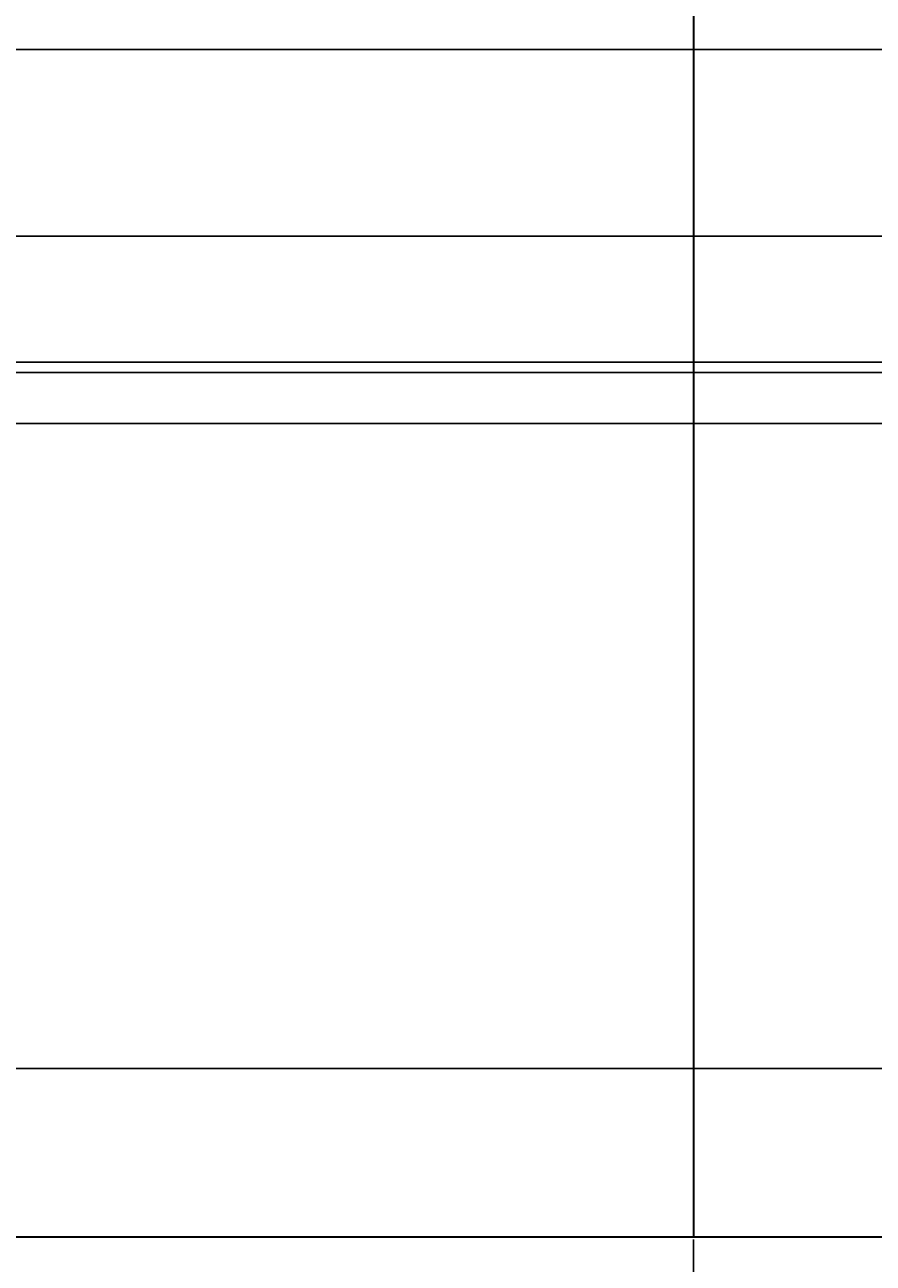
# Model space of a CAD drawing. Units: inches. Extents: x 27 to 200, y -50 to 102.
# Tile 4 of 26: x 67 to 89, y -17 to 15. Entities that reach past the tile are written whole.
import ezdxf

# ---------------------------------------------------------------- set-up
doc = ezdxf.new("R2010")
doc.units = ezdxf.units.IN
doc.header["$MEASUREMENT"] = 0
doc.layers.add('A-ANNO-DIMS', color=2, linetype='Continuous', lineweight=18)
doc.layers.add('A-ELEV', color=7, linetype='Continuous', lineweight=35)
doc.styles.get("Standard").update_dxf_attribs({"font": 'arial.ttf'})
doc.dimstyles.get("Standard").update_dxf_attribs({"dimtxt": 0.18, "dimasz": 0.18, "dimexe": 0.18, "dimexo": 0.0625, "dimgap": 0.09, "dimtad": 0, "dimtih": 1, "dimtoh": 1, "dimdec": 4, "dimzin": 0, "dimdsep": 46, "dimtxsty": 'Standard', "dimcen": 0.09, "dimadec": 0, "dimazin": 0, "dimtfac": 1, "dimtdec": 4, "dimtofl": 0, "dimtmove": 0, "dimatfit": 3, "dimfxl": 1, "dimtolj": 1, "dimtzin": 0, "dimarcsym": 0})

# ---------------------------------------------------------------- blocks, each defined once
blk = doc.blocks.new('*D23')
at = {"layer": 'A-ANNO-DIMS', "color": 0, "lineweight": -2, "transparency": 16777216}
for p, q in [((35.417, -16.832), (35.417, -25.149)), ((191.417, -16.832), (191.417, -25.149)), ((35.597, -24.969), (113.137, -24.969)), ((191.237, -24.969), (113.697, -24.969))]:
    blk.add_line(p, q, dxfattribs=at)
at = {"layer": 'A-ANNO-DIMS', "color": 0, "transparency": 16777216}
for points in [[(35.597, -24.939), (35.597, -24.999), (35.417, -24.969)], [(191.237, -24.939), (191.237, -24.999), (191.417, -24.969)]]:
    blk.add_solid(points, dxfattribs=at)
at = {"layer": 'Defpoints', "color": 0, "transparency": 16777216}
for p in [(35.417, -16.769), (191.417, -16.769), (191.417, -24.969)]:
    blk.add_point(p, dxfattribs=at)
at = {"layer": 'A-ANNO-DIMS', "color": 0, "transparency": 16777216, "insert": (113.417, -24.969), "char_height": 0.18, "attachment_point": 5}
blk.add_mtext('\\A1;156', dxfattribs=at)
blk = doc.blocks.new('*D33')
at = {"layer": 'A-ANNO-DIMS', "color": 0, "lineweight": -2, "transparency": 16777216}
for p, q in [((84.417, -16.832), (84.417, -25.149)), ((89.312, -16.832), (89.312, -25.149)), ((84.597, -24.969), (86.466, -24.969)), ((89.132, -24.969), (87.262, -24.969))]:
    blk.add_line(p, q, dxfattribs=at)
at = {"layer": 'A-ANNO-DIMS', "color": 0, "transparency": 16777216}
for points in [[(84.597, -24.939), (84.597, -24.999), (84.417, -24.969)], [(89.132, -24.939), (89.132, -24.999), (89.312, -24.969)]]:
    blk.add_solid(points, dxfattribs=at)
at = {"layer": 'Defpoints', "color": 0, "transparency": 16777216}
for p in [(84.417, -16.769), (89.312, -16.769), (89.312, -24.969)]:
    blk.add_point(p, dxfattribs=at)
at = {"layer": 'A-ANNO-DIMS', "color": 0, "transparency": 16777216, "insert": (86.864, -24.969), "char_height": 0.18, "attachment_point": 5}
blk.add_mtext('\\A1;4.895', dxfattribs=at)
blk = doc.blocks.new('*D43')
at = {"layer": 'A-ANNO-DIMS', "color": 0, "lineweight": -2, "transparency": 16777216}
for p, q in [((66.479, -3.679), (66.479, -25.149)), ((84.417, -16.832), (84.417, -25.149)), ((66.659, -24.969), (75.063, -24.969)), ((84.237, -24.969), (75.833, -24.969))]:
    blk.add_line(p, q, dxfattribs=at)
at = {"layer": 'A-ANNO-DIMS', "color": 0, "transparency": 16777216}
for points in [[(66.659, -24.939), (66.659, -24.999), (66.479, -24.969)], [(84.237, -24.939), (84.237, -24.999), (84.417, -24.969)]]:
    blk.add_solid(points, dxfattribs=at)
at = {"layer": 'Defpoints', "color": 0, "transparency": 16777216}
for p in [(66.479, -3.617), (84.417, -16.769), (84.417, -24.969)]:
    blk.add_point(p, dxfattribs=at)
at = {"layer": 'A-ANNO-DIMS', "color": 0, "transparency": 16777216, "insert": (75.448, -24.969), "char_height": 0.18, "attachment_point": 5}
blk.add_mtext('\\A1;17.94', dxfattribs=at)
blk = doc.blocks.new('*D48')
at = {"layer": 'A-ANNO-DIMS', "color": 0, "lineweight": -2, "transparency": 16777216}
for p, q in [((84.479, 44.926), (199.797, 44.926)), ((199.617, 44.746), (199.617, 14.26)), ((199.617, -16.589), (199.617, 13.897)), ((84.479, -16.769), (199.797, -16.769))]:
    blk.add_line(p, q, dxfattribs=at)
at = {"layer": 'A-ANNO-DIMS', "color": 0, "transparency": 16777216}
for points in [[(199.587, 44.746), (199.647, 44.746), (199.617, 44.926)], [(199.587, -16.589), (199.647, -16.589), (199.617, -16.769)]]:
    blk.add_solid(points, dxfattribs=at)
at = {"layer": 'Defpoints', "color": 0, "transparency": 16777216}
for p in [(84.417, 44.926), (199.617, 44.926), (84.417, -16.769)]:
    blk.add_point(p, dxfattribs=at)
at = {"layer": 'A-ANNO-DIMS', "color": 0, "transparency": 16777216, "insert": (199.617, 14.079), "char_height": 0.18, "attachment_point": 5}
blk.add_mtext('\\A1;61.7', dxfattribs=at)
blk = doc.blocks.new('*D54')
at = {"layer": 'A-ANNO-DIMS', "color": 0, "lineweight": -2, "transparency": 16777216}
for p, q in [((120.833, 13.977), (27.037, 13.977)), ((27.217, 13.797), (27.217, 11.743)), ((27.217, 9.324), (27.217, 11.379)), ((120.833, 9.144), (27.037, 9.144))]:
    blk.add_line(p, q, dxfattribs=at)
at = {"layer": 'A-ANNO-DIMS', "color": 0, "transparency": 16777216}
for points in [[(27.187, 13.797), (27.247, 13.797), (27.217, 13.977)], [(27.187, 9.324), (27.247, 9.324), (27.217, 9.144)]]:
    blk.add_solid(points, dxfattribs=at)
at = {"layer": 'Defpoints', "color": 0, "transparency": 16777216}
for p in [(27.217, 13.977), (120.895, 13.977), (120.895, 9.144)]:
    blk.add_point(p, dxfattribs=at)
at = {"layer": 'A-ANNO-DIMS', "color": 0, "transparency": 16777216, "insert": (27.217, 11.561), "char_height": 0.18, "attachment_point": 5}
blk.add_mtext('\\A1;4.83', dxfattribs=at)
blk = doc.blocks.new('*D56')
at = {"layer": 'A-ANNO-DIMS', "color": 0, "lineweight": -2, "transparency": 16777216}
for p, q in [((121.225, 5.878), (27.037, 5.878)), ((27.217, 5.698), (27.217, -3.085)), ((27.217, -12.231), (27.217, -3.448)), ((121.225, -12.411), (27.037, -12.411))]:
    blk.add_line(p, q, dxfattribs=at)
at = {"layer": 'A-ANNO-DIMS', "color": 0, "transparency": 16777216}
for points in [[(27.187, 5.698), (27.247, 5.698), (27.217, 5.878)], [(27.187, -12.231), (27.247, -12.231), (27.217, -12.411)]]:
    blk.add_solid(points, dxfattribs=at)
at = {"layer": 'Defpoints', "color": 0, "transparency": 16777216}
for p in [(27.217, 5.878), (121.288, 5.878), (121.288, -12.411)]:
    blk.add_point(p, dxfattribs=at)
at = {"layer": 'A-ANNO-DIMS', "color": 0, "transparency": 16777216, "insert": (27.217, -3.267), "char_height": 0.18, "attachment_point": 5}
blk.add_mtext('\\A1;18.29', dxfattribs=at)
blk = doc.blocks.new('*D68')
at = {"layer": 'A-ANNO-DIMS', "color": 0, "lineweight": -2, "transparency": 16777216}
for p, q in [((145.153, 5.617), (27.037, 5.617)), ((27.217, 5.437), (27.217, 5.138)), ((27.217, 4.476), (27.217, 4.774)), ((145.153, 4.296), (27.037, 4.296))]:
    blk.add_line(p, q, dxfattribs=at)
at = {"layer": 'A-ANNO-DIMS', "color": 0, "transparency": 16777216}
for points in [[(27.187, 5.437), (27.247, 5.437), (27.217, 5.617)], [(27.187, 4.476), (27.247, 4.476), (27.217, 4.296)]]:
    blk.add_solid(points, dxfattribs=at)
at = {"layer": 'Defpoints', "color": 0, "transparency": 16777216}
for p in [(27.217, 5.617), (145.216, 5.617), (145.216, 4.296)]:
    blk.add_point(p, dxfattribs=at)
at = {"layer": 'A-ANNO-DIMS', "color": 0, "transparency": 16777216, "insert": (27.217, 4.956), "char_height": 0.18, "attachment_point": 5}
blk.add_mtext('\\A1;1.32', dxfattribs=at)
blk = doc.blocks.new('*D69')
at = {"layer": 'A-ANNO-DIMS', "color": 0, "lineweight": -2, "transparency": 16777216}
for p, q in [((121.225, -12.411), (27.037, -12.411)), ((27.217, -12.591), (27.217, -14.408)), ((27.217, -16.589), (27.217, -14.772)), ((119.249, -16.769), (27.037, -16.769))]:
    blk.add_line(p, q, dxfattribs=at)
at = {"layer": 'A-ANNO-DIMS', "color": 0, "transparency": 16777216}
for points in [[(27.187, -12.591), (27.247, -12.591), (27.217, -12.411)], [(27.187, -16.589), (27.247, -16.589), (27.217, -16.769)]]:
    blk.add_solid(points, dxfattribs=at)
at = {"layer": 'Defpoints', "color": 0, "transparency": 16777216}
for p in [(27.217, -12.411), (121.288, -12.411), (119.312, -16.769)]:
    blk.add_point(p, dxfattribs=at)
at = {"layer": 'A-ANNO-DIMS', "color": 0, "transparency": 16777216, "insert": (27.217, -14.59), "char_height": 0.18, "attachment_point": 5}
blk.add_mtext('\\A1;4.358', dxfattribs=at)

msp = doc.modelspace()

# ---------------------------------------------------------------- linework, layer by layer
at = {"layer": 'A-ELEV'}
for p, q in [((84.4169, 44.9264), (84.4169, -16.7693)), ((35.4169, -16.7693), (191.4169, -16.7693))]:
    msp.add_line(p, q, dxfattribs=at)

# ---------------------------------------------------------------- dimensions: what is measured, and where the dimension line sits
at = {"layer": 'A-ANNO-DIMS'}
for base, p1, p2, override, picture, middle in [((199.6169, 44.9264), (84.4169, -16.7693), (84.4169, 44.9264), {"dimdec": 1, "dimlfac": 1, "dimrnd": 0, "dimzin": 0, "dimdsep": 46, "dimlunit": 2}, '*D48', (199.6169, 14.0786)), ((27.2169, 13.9773), (120.8954, 9.1438), (120.8954, 13.9773), {"dimdec": 2, "dimlfac": 1, "dimrnd": 0, "dimzin": 0, "dimdsep": 46, "dimlunit": 2}, '*D54', (27.2169, 11.5606)), ((27.2169, 5.8779), (121.2876, -12.411), (121.2876, 5.8779), {"dimdec": 2, "dimlfac": 1, "dimrnd": 0, "dimzin": 0, "dimdsep": 46, "dimlunit": 2}, '*D56', (27.2169, -3.2665)), ((27.2169, 5.6167), (145.216, 4.2959), (145.216, 5.6167), {"dimdec": 2, "dimlfac": 1, "dimrnd": 0, "dimzin": 0, "dimdsep": 46, "dimlunit": 2}, '*D68', (27.2169, 4.9563)), ((27.2169, -12.411), (119.3118, -16.7693), (121.2876, -12.411), {"dimdec": 3, "dimlfac": 1, "dimrnd": 0, "dimzin": 0, "dimdsep": 46, "dimlunit": 2}, '*D69', (27.2169, -14.5901))]:
    dim = msp.add_linear_dim(base=base, p1=p1, p2=p2, angle=90, dimstyle='Standard', override=override, dxfattribs=at)
    dim.commit()
    dim.dimension.update_dxf_attribs({"geometry": picture, "text_midpoint": middle})
for base, p1, p2, override, picture, middle in [((84.4169, -24.9693), (66.4786, -3.6168), (84.4169, -16.7693), {"dimdec": 2, "dimlfac": 1, "dimrnd": 0, "dimzin": 0, "dimdsep": 46, "dimlunit": 2}, '*D43', (75.4478, -24.9693)), ((191.4169, -24.9693), (35.4169, -16.7693), (191.4169, -16.7693), {"dimdec": 0, "dimlfac": 1, "dimrnd": 0, "dimzin": 0, "dimdsep": 46, "dimlunit": 2}, '*D23', (113.4169, -24.9693)), ((89.3118, -24.9693), (84.4169, -16.7693), (89.3118, -16.7693), {"dimdec": 3, "dimlfac": 1, "dimrnd": 0, "dimzin": 0, "dimdsep": 46, "dimlunit": 2}, '*D33', (86.8644, -24.9693))]:
    dim = msp.add_linear_dim(base=base, p1=p1, p2=p2, dimstyle='Standard', override=override, dxfattribs=at)
    dim.commit()
    dim.dimension.update_dxf_attribs({"geometry": picture, "text_midpoint": middle})

doc.saveas('drawing.dxf')
